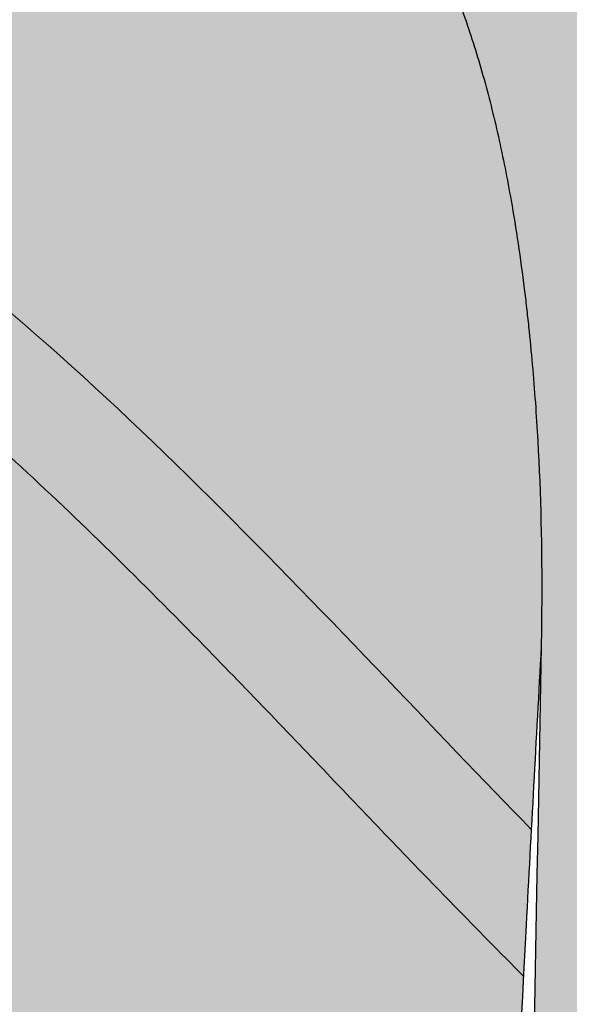
# Model space of a CAD drawing. Units: millimetres. Extents: x 11032 to 26788, y 3406 to 24505.
# Tile 60 of 78: x 16786 to 17293, y 16019 to 16927. Entities that reach past the tile are written whole.
import ezdxf

# ---------------------------------------------------------------- set-up
doc = ezdxf.new("R2010")
doc.units = ezdxf.units.MM
doc.header["$MEASUREMENT"] = 0
for name, color, linetype, lineweight in [('A-ANNO-DIMS', 2, 'Continuous', 18), ('A-ROOF', 7, 'Continuous', 30), ('E-LITE', 7, 'Continuous', 18), ('E-LITE-PATT', 7, 'Continuous', 13)]:
    doc.layers.add(name, color=color, linetype=linetype, lineweight=lineweight)
doc.layers.add('A-ROOF-PATT', color=9, linetype='Continuous', lineweight=13, true_color=0xc7c8ca)
doc.styles.get("Standard").update_dxf_attribs({"font": 'arial.ttf'})
doc.dimstyles.get("Standard").update_dxf_attribs({"dimtxt": 150, "dimasz": 100, "dimexe": 10, "dimexo": 5, "dimgap": 5, "dimtad": 0, "dimtih": 1, "dimtoh": 1, "dimdec": 0, "dimzin": 0, "dimdsep": 46, "dimtxsty": 'Standard', "dimcen": 0.09, "dimadec": 0, "dimazin": 0, "dimtfac": 1, "dimtdec": 0, "dimtofl": 0, "dimtmove": 0, "dimatfit": 3, "dimfxl": 1, "dimtolj": 1, "dimtzin": 0, "dimarcsym": 0})

# ---------------------------------------------------------------- blocks, each defined once
blk = doc.blocks.new('*D36')
at = {"layer": 'A-ANNO-DIMS', "color": 0, "lineweight": -2, "transparency": 16777216}
for p, q in [((12301.26, 17115.89), (12301.26, 24416.86)), ((25397.4, 4466.4), (25397.4, 24416.86)), ((12401.26, 24406.86), (18569.2, 24406.86)), ((25297.4, 24406.86), (19129.47, 24406.86))]:
    blk.add_line(p, q, dxfattribs=at)
at = {"layer": 'A-ANNO-DIMS', "color": 0, "transparency": 16777216}
for points in [[(12401.26, 24423.52), (12401.26, 24390.19), (12301.26, 24406.86)], [(25297.4, 24423.52), (25297.4, 24390.19), (25397.4, 24406.86)]]:
    blk.add_solid(points, dxfattribs=at)
at = {"layer": 'Defpoints', "color": 0, "transparency": 16777216}
for p in [(25397.4, 24406.86), (12301.26, 17110.89), (25397.4, 4461.4)]:
    blk.add_point(p, dxfattribs=at)
at = {"layer": 'A-ANNO-DIMS', "color": 0, "transparency": 16777216, "insert": (18849.33, 24406.86), "char_height": 150, "attachment_point": 5}
blk.add_mtext('\\A1;13096', dxfattribs=at)
blk = doc.blocks.new('*D37')
at = {"layer": 'A-ANNO-DIMS', "color": 0, "lineweight": -2, "transparency": 16777216}
for p, q in [((18087.74, 23450.36), (11334.76, 23450.36)), ((11344.76, 23350.36), (11344.76, 14037.46)), ((11344.76, 4561.4), (11344.76, 13874.29)), ((12927.66, 4461.4), (11334.76, 4461.4))]:
    blk.add_line(p, q, dxfattribs=at)
at = {"layer": 'A-ANNO-DIMS', "color": 0, "transparency": 16777216}
for points in [[(11328.1, 23350.36), (11361.43, 23350.36), (11344.76, 23450.36)], [(11328.1, 4561.4), (11361.43, 4561.4), (11344.76, 4461.4)]]:
    blk.add_solid(points, dxfattribs=at)
at = {"layer": 'Defpoints', "color": 0, "transparency": 16777216}
for p in [(11344.76, 23450.36), (18092.74, 23450.36), (12932.66, 4461.4)]:
    blk.add_point(p, dxfattribs=at)
at = {"layer": 'A-ANNO-DIMS', "color": 0, "transparency": 16777216, "insert": (11344.76, 13955.88), "char_height": 150, "attachment_point": 5}
blk.add_mtext('\\A1;18989', dxfattribs=at)
blk = doc.blocks.new('*D45')
at = {"layer": 'A-ANNO-DIMS', "color": 0, "lineweight": -2, "transparency": 16777216}
for p, q in [((13792.37, 18518.92), (26363.9, 18518.92)), ((26353.9, 18418.92), (26353.9, 17450.32)), ((26353.9, 16318.44), (26353.9, 17287.05)), ((22902.4, 16218.44), (26363.9, 16218.44))]:
    blk.add_line(p, q, dxfattribs=at)
at = {"layer": 'A-ANNO-DIMS', "color": 0, "transparency": 16777216}
for points in [[(26337.24, 18418.92), (26370.57, 18418.92), (26353.9, 18518.92)], [(26337.24, 16318.44), (26370.57, 16318.44), (26353.9, 16218.44)]]:
    blk.add_solid(points, dxfattribs=at)
at = {"layer": 'Defpoints', "color": 0, "transparency": 16777216}
for p in [(13787.37, 18518.92), (26353.9, 18518.92), (22897.4, 16218.44)]:
    blk.add_point(p, dxfattribs=at)
at = {"layer": 'A-ANNO-DIMS', "color": 0, "transparency": 16777216, "insert": (26353.9, 17368.68), "char_height": 150, "attachment_point": 5}
blk.add_mtext('\\A1;2300.5', dxfattribs=at)
blk = doc.blocks.new('*D57')
at = {"layer": 'A-ANNO-DIMS', "color": 0, "lineweight": -2, "transparency": 16777216}
for p, q in [((14994.7, 7266.4), (14994.7, 24416.86)), ((20894.7, 7266.4), (20894.7, 24416.86)), ((15094.7, 24406.86), (17715.98, 24406.86)), ((20794.7, 24406.86), (18173.42, 24406.86))]:
    blk.add_line(p, q, dxfattribs=at)
at = {"layer": 'A-ANNO-DIMS', "color": 0, "transparency": 16777216}
for points in [[(15094.7, 24423.52), (15094.7, 24390.19), (14994.7, 24406.86)], [(20794.7, 24423.52), (20794.7, 24390.19), (20894.7, 24406.86)]]:
    blk.add_solid(points, dxfattribs=at)
at = {"layer": 'Defpoints', "color": 0, "transparency": 16777216}
for p in [(20894.7, 24406.86), (14994.7, 7261.4), (20894.7, 7261.4)]:
    blk.add_point(p, dxfattribs=at)
at = {"layer": 'A-ANNO-DIMS', "color": 0, "transparency": 16777216, "insert": (17944.7, 24406.86), "char_height": 150, "attachment_point": 5}
blk.add_mtext('\\A1;5900', dxfattribs=at)

msp = doc.modelspace()

# ---------------------------------------------------------------- hatches: boundary and pattern name
at = {"layer": 'A-ROOF-PATT'}
h = msp.add_hatch(color=256, dxfattribs=at)
edge = h.paths.add_edge_path()
edge.add_spline(control_points=[(17532.827, 17324.837), (17391.335, 17349.016), (16840.872, 17494.912), (16080.055, 18069.544), (14738.803, 18299.641), (13382.429, 18838.336), (12580.532, 17870.207), (12430.422, 17563.822)], knot_values=[2977.6027945, 2977.6027945, 2977.6027945, 2977.6027945, 3438.1840601, 4811.6463022, 5622.8675483, 7588.0288188, 8560.6685791, 8560.6685791, 8560.6685791, 8560.6685791], degree=3, periodic=0)
edge.add_spline(control_points=[(12430.422, 17563.822), (12437.904, 17573.36), (12445.386, 17582.899), (12452.869, 17592.437), (12452.869, 17592.438), (12452.869, 17592.438), (12452.869, 17592.438)], knot_values=[1408.564138, 1408.564138, 1408.564138, 1408.564138, 1444.85989, 1444.85989, 1444.85989, 1444.8601183, 1444.8601183, 1444.8601183, 1444.8601183], degree=3, periodic=0)
edge.add_spline(control_points=[(12452.869, 17592.438), (12555.432, 17723.185), (12736.557, 17929.686), (13044.86, 18114.643), (13219.943, 18189.644), (13299.92, 18220.646)], knot_values=[339.318246, 339.318246, 339.318246, 339.318246, 836.8349967, 1151.2512933, 1408.564138, 1408.564138, 1408.564138, 1408.564138], degree=3, periodic=0)
edge.add_spline(control_points=[(13299.92, 18220.646), (13299.998, 18220.689), (13300.077, 18220.732), (13319.738, 18231.488), (13339.24, 18241.402), (13388.645, 18264.703), (13418.466, 18277.069), (13478.019, 18298.648), (13507.751, 18307.861), (13544.561, 18317.488), (13551.584, 18319.245), (13558.612, 18320.924)], knot_values=[3783.8950972, 3783.8950972, 3783.8950972, 3783.8950972, 3784.1737101, 3784.1737101, 3853.4666747, 3853.4666747, 3960.2401917, 3960.2401917, 4067.0137087, 4067.0137087, 4092.1744649, 4092.1744649, 4092.1744649, 4092.1744649], degree=3, periodic=0)
edge.add_spline(control_points=[(13558.612, 18320.924), (13581.407, 18326.373), (13604.25, 18331.007), (13657.184, 18339.957), (13687.338, 18343.732), (13748.098, 18348.892), (13778.704, 18350.276), (13840.46, 18350.833), (13871.609, 18350.005), (13934.496, 18346.313), (13966.232, 18343.449), (14030.297, 18335.871), (14062.625, 18331.158), (14127.853, 18320.088), (14160.753, 18313.73), (14241.357, 18296.556), (14289.343, 18284.997), (14386.31, 18259.688), (14435.291, 18245.941), (14534.161, 18217.034), (14584.049, 18201.875), (14684.682, 18170.964), (14735.427, 18155.212), (14837.763, 18123.971), (14889.354, 18108.482), (14954.971, 18089.677), (14968.586, 18085.823), (14992.391, 18079.184), (15002.566, 18076.376), (15021.739, 18071.153), (15030.731, 18068.729), (15047.707, 18064.21), (15055.694, 18062.106), (15079.815, 18055.825), (15095.905, 18051.728), (15143.966, 18039.717), (15175.729, 18032.084), (15254.84, 18013.501), (15301.798, 18002.866), (15394.186, 17981.845), (15439.615, 17971.459), (15528.833, 17950.135), (15572.62, 17939.197), (15658.477, 17916.021), (15700.546, 17903.785), (15753.633, 17886.734), (15765.446, 17882.835), (15786.574, 17875.653), (15795.915, 17872.404), (15810.108, 17867.349), (15814.99, 17865.588), (15824.736, 17862.029), (15829.611, 17860.226), (15844.241, 17854.75), (15854.002, 17851.008), (15883.312, 17839.521), (15902.885, 17831.512), (15966.355, 17804.548), (16010.39, 17784.302), (16098.838, 17741.267), (16143.25, 17718.478), (16232.497, 17671.098), (16277.332, 17646.507), (16367.515, 17596.295), (16412.862, 17570.676), (16504.202, 17519.209), (16550.194, 17493.362), (16643.009, 17442.263), (16689.831, 17417.011), (16756.517, 17382.472), (16775.937, 17372.58), (16795.455, 17362.84)], knot_values=[4092.1744649, 4092.1744649, 4092.1744649, 4092.1744649, 4173.7872258, 4173.7872258, 4280.5607428, 4280.5607428, 4387.3342598, 4387.3342598, 4494.1077768, 4494.1077768, 4600.8812939, 4600.8812939, 4707.6548109, 4707.6548109, 4814.4283279, 4814.4283279, 4967.1262405, 4967.1262405, 5119.8241531, 5119.8241531, 5272.5220657, 5272.5220657, 5425.2199783, 5425.2199783, 5577.9178908, 5577.9178908, 5617.7853319, 5617.7853319, 5647.4648479, 5647.4648479, 5673.611025, 5673.611025, 5696.747607, 5696.747607, 5743.6818903, 5743.6818903, 5837.5504571, 5837.5504571, 5979.7261046, 5979.7261046, 6121.9017521, 6121.9017521, 6264.0773996, 6264.0773996, 6406.2530471, 6406.2530471, 6447.2585849, 6447.2585849, 6480.0420882, 6480.0420882, 6497.3077062, 6497.3077062, 6514.5733242, 6514.5733242, 6549.1045602, 6549.1045602, 6618.1670322, 6618.1670322, 6772.6610171, 6772.6610171, 6927.155002, 6927.155002, 7081.6489869, 7081.6489869, 7236.1429718, 7236.1429718, 7390.6369567, 7390.6369567, 7545.1309416, 7545.1309416, 7608.1992868, 7608.1992868, 7608.1992868, 7608.1992868], degree=3, periodic=0)
edge.add_spline(control_points=[(16795.455, 17362.84), (16814.335, 17349.456), (16832.897, 17336.263), (16873.225, 17307.197), (16894.778, 17291.386), (16936.221, 17259.941), (16956.11, 17244.308), (16993.863, 17213.094), (17011.726, 17197.514), (17041.993, 17169.265), (17054.791, 17156.601), (17078.762, 17131.225), (17089.933, 17118.516), (17110.618, 17092.991), (17120.131, 17080.178), (17130.17, 17065.264), (17131.487, 17063.277), (17133.77, 17059.776), (17134.746, 17058.261), (17136.69, 17055.205), (17137.657, 17053.668), (17140.539, 17049.025), (17142.438, 17045.89), (17148.068, 17036.367), (17151.732, 17029.859), (17163.03, 17008.788), (17170.335, 16993.646), (17184.087, 16961.978), (17190.534, 16945.453), (17202.562, 16911.165), (17208.142, 16893.402), (17218.448, 16856.821), (17223.173, 16838.003), (17231.801, 16799.51), (17235.705, 16779.837), (17241.533, 16746.739), (17243.676, 16733.5), (17247.718, 16706.37), (17249.608, 16692.472), (17252.066, 16672.69), (17252.761, 16666.875), (17254.1, 16655.226), (17254.744, 16649.4), (17256.596, 16631.917), (17257.727, 16620.254), (17260.823, 16585.238), (17262.489, 16561.858), (17266.551, 16488.654), (17267.658, 16438.661), (17267.349, 16375.228), (17267.193, 16362.07), (17266.95, 16348.891)], knot_values=[15.1130472, 15.1130472, 15.1130472, 15.1130472, 82.6995146, 82.6995146, 165.3990291, 165.3990291, 248.0985437, 248.0985437, 330.7980583, 330.7980583, 397.9419458, 397.9419458, 465.0858333, 465.0858333, 532.2297209, 532.2297209, 542.533741, 542.533741, 550.3568158, 550.3568158, 558.1798906, 558.1798906, 573.8260402, 573.8260402, 605.1183395, 605.1183395, 672.7640614, 672.7640614, 740.4097834, 740.4097834, 808.0555054, 808.0555054, 875.7012273, 875.7012273, 943.3469493, 943.3469493, 987.6613492, 987.6613492, 1033.4121612, 1033.4121612, 1052.3850876, 1052.3850876, 1071.358014, 1071.358014, 1109.3038668, 1109.3038668, 1185.1955724, 1185.1955724, 1346.4419026, 1346.4419026, 1388.5586631, 1388.5586631, 1388.5586631, 1388.5586631], degree=3, periodic=0)
edge.add_spline(control_points=[(17266.95, 16348.891), (17266.95, 16348.891), (17266.95, 16348.891), (17266.95, 16348.891), (17253.182, 15602.417), (17239.414, 14855.943), (17225.646, 14109.469)], knot_values=[1388.5586631, 1388.5586631, 1388.5586631, 1388.5586631, 1388.5589654, 1388.5589654, 1388.5589654, 3774.0767661, 3774.0767661, 3774.0767661, 3774.0767661], degree=3, periodic=0)
edge.add_spline(control_points=[(17225.646, 14109.469), (17226.198, 14109.827), (17226.748, 14110.185), (17242.065, 14120.191), (17255.956, 14130.116), (17274.422, 14144.286), (17279.609, 14148.386), (17284.686, 14152.511)], knot_values=[1926.3423968, 1926.3423968, 1926.3423968, 1926.3423968, 1927.316729, 1927.316729, 1953.5121761, 1953.5121761, 1964.0732348, 1964.0732348, 1964.0732348, 1964.0732348], degree=3, periodic=0)
edge.add_spline(control_points=[(17284.686, 14152.511), (17315.791, 14194.761), (17384.413, 14446.273), (17407.128, 14793.401), (17407.093, 15295.84), (17423.274, 15626.362), (17415.601, 15782.507)], knot_values=[0, 0, 0, 0, 163.2554674, 619.2296767, 1171.8624483, 1621.6355562, 1621.6355562, 1621.6355562, 1621.6355562], degree=3, periodic=0)
edge.add_spline(control_points=[(17415.601, 15782.507), (17438.21, 16077.57), (17410.495, 16533.484), (17390.893, 17030.649), (17301.082, 17169.349)], knot_values=[543.9784753, 543.9784753, 543.9784753, 543.9784753, 1452.9852767, 1960.0114926, 1960.0114926, 1960.0114926, 1960.0114926], degree=3, periodic=0)
edge.add_spline(control_points=[(17301.082, 17169.349), (17346.58, 17157.64), (17392.235, 17147.336), (17467.161, 17132.609), (17496.336, 17127.412), (17525.58, 17122.709)], knot_values=[8131.593939, 8131.593939, 8131.593939, 8131.593939, 8269.7349273, 8269.7349273, 8357.5016646, 8357.5016646, 8357.5016646, 8357.5016646], degree=3, periodic=0)
edge.add_line((17525.58, 17122.709), (17532.827, 17324.837))
edge = h.paths.add_edge_path(flags=17)
edge.add_spline(control_points=[(13340.537, 14602.706), (13316.172, 14726.456), (13323.666, 14932.342), (13637.836, 15081.117), (13863.248, 15171.051), (14002.1, 15224.503), (14058.539, 15244.876)], knot_values=[680.8931862, 680.8931862, 680.8931862, 680.8931862, 1033.4728289, 1337.4008326, 1604.7214264, 1784.2944722, 1784.2944722, 1784.2944722, 1784.2944722], degree=3, periodic=0)
edge.add_spline(control_points=[(14058.539, 15244.876), (14058.289, 15275.236), (14057.634, 15305.434), (14055.312, 15376.527), (14053.359, 15417.248), (14048.642, 15497.048), (14045.89, 15536.143), (14042.888, 15574.619)], knot_values=[6573.1065419, 6573.1065419, 6573.1065419, 6573.1065419, 6636.7330012, 6636.7330012, 6723.8890547, 6723.8890547, 6809.6328771, 6809.6328771, 6809.6328771, 6809.6328771], degree=3, periodic=0)
edge.add_spline(control_points=[(14042.888, 15574.619), (13546.54, 15403.221), (13074.735, 15143.241), (13277.36, 14695.339), (13340.537, 14602.706)], knot_values=[503.7925783, 503.7925783, 503.7925783, 503.7925783, 1728.1787606, 2051.34844, 2051.34844, 2051.34844, 2051.34844], degree=3, periodic=0)
h = msp.add_hatch(color=256, dxfattribs=at)
h.set_gradient(color1=(254, 234, 185), color2=(254, 204, 102), name='HEMISPHERICAL')
edge = h.paths.add_edge_path()
edge.add_line((15084.393, 17001.32), (15284.393, 17051.32))
edge.add_line((15284.393, 17051.32), (15470.537, 16752.334))
edge.add_spline(control_points=[(15470.537, 16752.334), (15683.311, 16831.508), (16106.827, 16912.335), (16625.609, 16876.997), (17083.498, 16357.78), (17257.801, 16180.113)], knot_values=[0, 0, 0, 0, 655.2936334, 1252.0157838, 1989.6162859, 1989.6162859, 1989.6162859, 1989.6162859], degree=3, periodic=0)
edge.add_spline(control_points=[(17257.801, 16180.113), (17260.851, 16236.372), (17263.9, 16292.632), (17266.95, 16348.891)], knot_values=[1132.9967717, 1132.9967717, 1132.9967717, 1132.9967717, 1198.0464225, 1198.0464225, 1198.0464225, 1198.0464225], degree=3, periodic=0)
edge.add_spline(control_points=[(17266.95, 16348.891), (17267.193, 16362.07), (17267.349, 16375.228), (17267.658, 16438.661), (17266.551, 16488.654), (17262.489, 16561.858), (17260.823, 16585.238), (17257.727, 16620.254), (17256.596, 16631.917), (17254.744, 16649.4), (17254.1, 16655.226), (17252.761, 16666.875), (17252.066, 16672.69), (17249.608, 16692.472), (17247.718, 16706.37), (17243.676, 16733.5), (17241.533, 16746.739), (17235.705, 16779.837), (17231.801, 16799.51), (17223.173, 16838.003), (17218.448, 16856.821), (17208.142, 16893.402), (17202.562, 16911.165), (17190.534, 16945.453), (17184.087, 16961.978), (17170.335, 16993.646), (17163.03, 17008.788), (17151.732, 17029.859), (17148.068, 17036.367), (17142.438, 17045.89), (17140.539, 17049.025), (17137.657, 17053.668), (17136.69, 17055.205), (17134.746, 17058.261), (17133.77, 17059.776), (17131.487, 17063.277), (17130.17, 17065.264), (17120.131, 17080.178), (17110.618, 17092.991), (17089.933, 17118.516), (17078.762, 17131.225), (17054.791, 17156.601), (17041.993, 17169.265), (17011.726, 17197.514), (16993.863, 17213.094), (16956.11, 17244.308), (16936.221, 17259.941), (16894.778, 17291.386), (16873.225, 17307.197), (16832.897, 17336.263), (16814.335, 17349.456), (16795.455, 17362.84)], knot_values=[15.1130472, 15.1130472, 15.1130472, 15.1130472, 57.2298077, 57.2298077, 218.4761379, 218.4761379, 294.3678435, 294.3678435, 332.3136963, 332.3136963, 351.2866227, 351.2866227, 370.2595491, 370.2595491, 416.0103612, 416.0103612, 460.324761, 460.324761, 527.970483, 527.970483, 595.616205, 595.616205, 663.2619269, 663.2619269, 730.9076489, 730.9076489, 798.5533709, 798.5533709, 829.8456701, 829.8456701, 845.4918197, 845.4918197, 853.3148945, 853.3148945, 861.1379693, 861.1379693, 871.4419895, 871.4419895, 938.585877, 938.585877, 1005.7297645, 1005.7297645, 1072.8736521, 1072.8736521, 1155.5731666, 1155.5731666, 1238.2726812, 1238.2726812, 1320.9721958, 1320.9721958, 1388.5586631, 1388.5586631, 1388.5586631, 1388.5586631], degree=3, periodic=0)
edge.add_spline(control_points=[(16795.455, 17362.84), (16775.937, 17372.58), (16756.517, 17382.472), (16689.831, 17417.011), (16643.009, 17442.263), (16550.194, 17493.362), (16504.202, 17519.209), (16412.862, 17570.676), (16367.515, 17596.295), (16277.332, 17646.507), (16232.497, 17671.098), (16143.25, 17718.478), (16098.838, 17741.267), (16010.39, 17784.302), (15966.355, 17804.548), (15902.885, 17831.512), (15883.312, 17839.521), (15854.002, 17851.008), (15844.241, 17854.75), (15829.611, 17860.226), (15824.736, 17862.029), (15814.99, 17865.588), (15810.108, 17867.349), (15795.915, 17872.404), (15786.574, 17875.653), (15765.446, 17882.835), (15753.633, 17886.734), (15700.546, 17903.785), (15658.477, 17916.021), (15572.62, 17939.197), (15528.833, 17950.135), (15439.615, 17971.459), (15394.186, 17981.845), (15301.798, 18002.866), (15254.84, 18013.501), (15175.729, 18032.084), (15143.966, 18039.717), (15095.905, 18051.728), (15079.815, 18055.825), (15055.694, 18062.106), (15047.707, 18064.21), (15030.731, 18068.729), (15021.739, 18071.153), (15002.566, 18076.376), (14992.391, 18079.184), (14968.586, 18085.823), (14954.971, 18089.677), (14889.354, 18108.482), (14837.763, 18123.971), (14735.427, 18155.212), (14684.682, 18170.964), (14584.049, 18201.875), (14534.161, 18217.034), (14435.291, 18245.941), (14386.31, 18259.688), (14289.343, 18284.997), (14241.357, 18296.556), (14160.753, 18313.73), (14127.853, 18320.088), (14062.625, 18331.158), (14030.297, 18335.871), (13966.232, 18343.449), (13934.496, 18346.313), (13871.609, 18350.005), (13840.46, 18350.833), (13778.704, 18350.276), (13748.098, 18348.892), (13687.338, 18343.732), (13657.184, 18339.957), (13604.25, 18331.007), (13581.407, 18326.373), (13558.612, 18320.924)], knot_values=[4092.1744649, 4092.1744649, 4092.1744649, 4092.1744649, 4155.2428101, 4155.2428101, 4309.736795, 4309.736795, 4464.2307799, 4464.2307799, 4618.7247648, 4618.7247648, 4773.2187497, 4773.2187497, 4927.7127346, 4927.7127346, 5082.2067195, 5082.2067195, 5151.2691915, 5151.2691915, 5185.8004275, 5185.8004275, 5203.0660455, 5203.0660455, 5220.3316635, 5220.3316635, 5253.1151668, 5253.1151668, 5294.1207046, 5294.1207046, 5436.2963521, 5436.2963521, 5578.4719996, 5578.4719996, 5720.6476471, 5720.6476471, 5862.8232946, 5862.8232946, 5956.6918614, 5956.6918614, 6003.6261447, 6003.6261447, 6026.7627267, 6026.7627267, 6052.9089038, 6052.9089038, 6082.5884198, 6082.5884198, 6122.4558609, 6122.4558609, 6275.1537734, 6275.1537734, 6427.851686, 6427.851686, 6580.5495986, 6580.5495986, 6733.2475112, 6733.2475112, 6885.9454238, 6885.9454238, 6992.7189408, 6992.7189408, 7099.4924578, 7099.4924578, 7206.2659749, 7206.2659749, 7313.0394919, 7313.0394919, 7419.8130089, 7419.8130089, 7526.5865259, 7526.5865259, 7608.1992868, 7608.1992868, 7608.1992868, 7608.1992868], degree=3, periodic=0)
edge.add_spline(control_points=[(13558.612, 18320.924), (13472.381, 18287.498), (13386.15, 18254.072), (13299.92, 18220.646), (13299.92, 18220.646), (13299.92, 18220.646), (13299.92, 18220.646)], knot_values=[61.8832457, 61.8832457, 61.8832457, 61.8832457, 339.3179746, 339.3179746, 339.3179746, 339.318246, 339.318246, 339.318246, 339.318246], degree=3, periodic=0)
edge.add_spline(control_points=[(13299.92, 18220.646), (13219.943, 18189.644), (13044.86, 18114.643), (12736.557, 17929.686), (12555.432, 17723.185), (12452.869, 17592.438)], knot_values=[339.318246, 339.318246, 339.318246, 339.318246, 596.6310906, 911.0473872, 1408.564138, 1408.564138, 1408.564138, 1408.564138], degree=3, periodic=0)
edge.add_spline(control_points=[(12452.869, 17592.438), (12452.869, 17592.438), (12452.869, 17592.438), (12452.869, 17592.437), (12445.386, 17582.899), (12437.904, 17573.36), (12430.422, 17563.822)], knot_values=[1408.564138, 1408.564138, 1408.564138, 1408.564138, 1408.5643663, 1408.5643663, 1408.5643663, 1444.8601183, 1444.8601183, 1444.8601183, 1444.8601183], degree=3, periodic=0)
edge.add_spline(control_points=[(12430.422, 17563.822), (12373.797, 17448.248), (12157.302, 16836.764), (12751.985, 16393.69), (13424.325, 15907.903), (14042.888, 15574.619)], knot_values=[0, 0, 0, 0, 366.8993034, 1975.5941082, 2977.6027945, 2977.6027945, 2977.6027945, 2977.6027945], degree=3, periodic=0)
edge.add_spline(control_points=[(14042.888, 15574.619), (14042.839, 15575.252), (14042.789, 15575.886), (14039.681, 15615.607), (14036.366, 15654.052), (14029.551, 15729.305), (14026.05, 15766.114), (14019.175, 15837.686), (14015.8, 15872.45), (13903.823, 16338.596)], knot_values=[6310.2261504, 6310.2261504, 6310.2261504, 6310.2261504, 6311.6383814, 6311.6383814, 6398.7944349, 6398.7944349, 6485.9504884, 6485.9504884, 6573.1065419, 6573.1065419, 6573.1065419, 6573.1065419], degree=3, periodic=0)
edge.add_spline(control_points=[(13903.823, 16338.596), (14237.315, 16236.889), (14456.623, 16167.555), (14614.196, 16115.84)], knot_values=[0, 0, 0, 0, 202.9853419, 202.9853419, 202.9853419, 202.9853419], degree=3, periodic=0)
edge.add_spline(control_points=[(14614.196, 16115.84), (14663.209, 16178.992), (14799.965, 16341.237), (14969.915, 16481.426), (15084.393, 16556.825)], knot_values=[2405.0345045, 2405.0345045, 2405.0345045, 2405.0345045, 2644.8826966, 3039.2707272, 3039.2707272, 3039.2707272, 3039.2707272], degree=3, periodic=0)
edge.add_line((15084.393, 16556.825), (15084.393, 17001.32))
h.paths.add_polyline_path([(14195.599, 17606.181, -1), (14395.599, 17606.181, -1)], flags=16)
h.paths.add_polyline_path([(13310.178, 17032.97, -1), (13510.178, 17032.97, -1)], flags=16)
h = msp.add_hatch(color=256, dxfattribs=at)
h.set_gradient(color1=(254, 234, 185), color2=(254, 204, 102), name='HEMISPHERICAL')
edge = h.paths.add_edge_path()
edge.add_spline(control_points=[(16560.042, 14907.752), (16569.192, 14907.664), (16578.343, 14907.575), (16587.493, 14907.486), (16832.101, 14905.115), (17122.895, 14902.296), (16849.359, 14976.117), (16870.954, 15304.114), (17098.337, 15241.178), (17235.385, 15203.245)], knot_values=[0, 0, 0, 0, 14.8674385, 14.8674385, 14.8674385, 412.2943091, 487.3345915, 708.6416004, 1044.3939449, 1044.3939449, 1044.3939449, 1044.3939449], degree=3, periodic=0)
edge.add_line((16587.504, 14907.486), (16560.207, 14907.486))
edge.add_line((16560.207, 14907.486), (15784.393, 16153.61))
edge.add_line((15784.393, 16153.61), (15784.393, 15385.996))
edge.add_spline(control_points=[(15784.393, 15385.996), (15798.391, 15360.52), (15847.198, 15266.214), (15887.196, 15168.614), (15912.903, 15096.727)], knot_values=[1463.2850479, 1463.2850479, 1463.2850479, 1463.2850479, 1550.659771, 1779.9599361, 1779.9599361, 1779.9599361, 1779.9599361], degree=3, periodic=0)
edge.add_spline(control_points=[(15912.903, 15096.727), (15913.652, 15095.649), (15914.403, 15094.565), (15925.191, 15078.948), (15935.516, 15063.47), (15956.582, 15030.918), (15967.324, 15013.844), (15989.119, 14978.386), (16000.173, 14960.003), (16022.525, 14922.193), (16033.824, 14902.767), (16056.63, 14863.116), (16068.138, 14842.891), (16091.349, 14801.871), (16103.053, 14781.075), (16126.666, 14739.118), (16138.575, 14717.958), (16162.628, 14675.459), (16174.772, 14654.12), (16199.352, 14611.428), (16211.787, 14590.075), (16237.037, 14547.491), (16249.851, 14526.26), (16271.946, 14490.566), (16281.092, 14476.044), (16299.694, 14447.129), (16309.149, 14432.737), (16328.456, 14404.098), (16338.307, 14389.85), (16358.518, 14361.503), (16368.879, 14347.403), (16390.266, 14319.347), (16401.291, 14305.391), (16420.626, 14281.969), (16428.703, 14272.467), (16445.363, 14253.527), (16453.946, 14244.088), (16471.727, 14225.278), (16480.926, 14215.907), (16500.075, 14197.247), (16510.026, 14187.959), (16530.844, 14169.504), (16541.71, 14160.337), (16564.549, 14142.195), (16576.522, 14133.22), (16597.69, 14118.448), (16606.528, 14112.565), (16624.87, 14101.004), (16634.376, 14095.326), (16654.117, 14084.255), (16664.352, 14078.862), (16685.603, 14068.46), (16696.619, 14063.452), (16719.46, 14053.944), (16731.285, 14049.444), (16755.742, 14041.097), (16768.374, 14037.251), (16794.396, 14030.368), (16807.787, 14027.332), (16835.229, 14022.23), (16849.279, 14020.163), (16877.882, 14017.141), (16892.435, 14016.186), (16921.835, 14015.489), (16936.683, 14015.749), (16961.564, 14017.241), (16971.582, 14018.127), (16986.57, 14019.883), (16991.56, 14020.54), (16999.027, 14021.63), (17001.514, 14022.011), (17006.48, 14022.809), (17008.962, 14023.225), (17014.824, 14024.251), (17018.193, 14024.875), (17036.262, 14028.398), (17050.55, 14031.826), (17078.171, 14039.583), (17091.505, 14043.912), (17115.643, 14052.705), (17126.557, 14057.089), (17137.108, 14061.688)], knot_values=[2010.7639617, 2010.7639617, 2010.7639617, 2010.7639617, 2014.7029827, 2014.7029827, 2067.238337, 2067.238337, 2119.7736913, 2119.7736913, 2172.3090457, 2172.3090457, 2224.8444, 2224.8444, 2277.3797543, 2277.3797543, 2329.9151086, 2329.9151086, 2382.450463, 2382.450463, 2434.9858173, 2434.9858173, 2487.5211716, 2487.5211716, 2540.0565259, 2540.0565259, 2576.3179289, 2576.3179289, 2612.5793318, 2612.5793318, 2648.8407347, 2648.8407347, 2685.1021376, 2685.1021376, 2721.3635405, 2721.3635405, 2746.252015, 2746.252015, 2771.1404895, 2771.1404895, 2796.028964, 2796.028964, 2820.9174385, 2820.9174385, 2845.8059131, 2845.8059131, 2870.6943876, 2870.6943876, 2887.5132757, 2887.5132757, 2904.3321639, 2904.3321639, 2921.1510521, 2921.1510521, 2937.9699402, 2937.9699402, 2954.7888284, 2954.7888284, 2971.6077166, 2971.6077166, 2988.4266047, 2988.4266047, 3005.2454929, 3005.2454929, 3022.0643811, 3022.0643811, 3038.8832692, 3038.8832692, 3050.1975453, 3050.1975453, 3055.8546833, 3055.8546833, 3058.6832524, 3058.6832524, 3061.5118214, 3061.5118214, 3065.3934173, 3065.3934173, 3082.4668716, 3082.4668716, 3099.5403259, 3099.5403259, 3114.5433443, 3114.5433443, 3114.5433443, 3114.5433443], degree=3, periodic=0)
edge.add_spline(control_points=[(17137.108, 14061.688), (17165.253, 14274.398), (17209.97, 14653.885), (17230.2, 15035.586), (17235.385, 15203.245)], knot_values=[1968.0804557, 1968.0804557, 1968.0804557, 1968.0804557, 2611.5282875, 3114.5379264, 3114.5379264, 3114.5379264, 3114.5379264], degree=3, periodic=0)
edge = h.paths.add_edge_path()
edge.add_spline(control_points=[(16856.103, 14956.992), (16852.841, 14961.219), (16849.83, 14965.576), (16842.539, 14977.287), (16838.658, 14984.798), (16832.033, 15000.109), (16829.289, 15007.911), (16824.126, 15026.008), (16822.047, 15036.354), (16819.308, 15057.097), (16818.649, 15067.496), (16818.576, 15088.188), (16819.162, 15098.483), (16821.467, 15118.823), (16823.186, 15128.868), (16827.696, 15148.567), (16830.486, 15158.22), (16836.065, 15173.969), (16838.565, 15180.211), (16844.079, 15192.402), (16847.092, 15198.353), (16852.029, 15207.021), (16853.744, 15209.868), (16857.321, 15215.468), (16859.188, 15218.226), (16863.017, 15223.558), (16864.978, 15226.136), (16872.565, 15235.558), (16878.593, 15241.952), (16891.428, 15253.591), (16898.232, 15258.834), (16912.397, 15268.127), (16919.756, 15272.176), (16934.816, 15279.138), (16942.515, 15282.052), (16958.1, 15286.873), (16965.985, 15288.78), (16984.013, 15292.142), (16994.186, 15293.334), (17014.631, 15294.619), (17024.904, 15294.713), (17048.453, 15293.935), (17061.76, 15292.783), (17088.519, 15289.422), (17101.972, 15287.211), (17131.961, 15281.46), (17148.526, 15277.734), (17181.692, 15269.627), (17198.292, 15265.245), (17222.182, 15258.759), (17229.535, 15256.737), (17236.862, 15254.714)], knot_values=[9.6639535, 9.6639535, 9.6639535, 9.6639535, 20.0351668, 20.0351668, 36.9411752, 36.9411752, 53.8471837, 53.8471837, 75.7795687, 75.7795687, 97.7119538, 97.7119538, 119.6443388, 119.6443388, 141.5767238, 141.5767238, 163.5091089, 163.5091089, 178.3829945, 178.3829945, 193.2568801, 193.2568801, 200.6938229, 200.6938229, 208.1307657, 208.1307657, 215.4448585, 215.4448585, 235.5795923, 235.5795923, 255.7143261, 255.7143261, 275.8490598, 275.8490598, 295.9837936, 295.9837936, 316.1185274, 316.1185274, 341.7220543, 341.7220543, 367.3255812, 367.3255812, 400.1572431, 400.1572431, 432.988905, 432.988905, 473.0440165, 473.0440165, 513.099128, 513.099128, 530.9692999, 530.9692999, 530.9692999, 530.9692999], degree=3, periodic=0)
edge.add_spline(control_points=[(17236.862, 15254.714), (17240.377, 15387.456), (17242.496, 15609.536), (17239.752, 15831.567), (17250.544, 16044.717)], knot_values=[1250.9818616, 1250.9818616, 1250.9818616, 1250.9818616, 1649.1516581, 1916.613987, 1916.613987, 1916.613987, 1916.613987], degree=3, periodic=0)
edge.add_spline(control_points=[(17250.544, 16044.717), (17229.169, 16066.505), (17207.794, 16088.292), (17186.419, 16110.08), (17186.418, 16110.08), (17186.418, 16110.081), (17186.418, 16110.081)], knot_values=[-88.5185581, -88.5185581, -88.5185581, -88.5185581, -0.0012784, -0.0012784, -0.0012784, 0, 0, 0, 0], degree=3, periodic=0)
edge.add_spline(control_points=[(17186.418, 16110.081), (17169.261, 16127.569), (17151.499, 16145.947), (17114.892, 16184.084), (17096.046, 16203.842), (17057.437, 16244.305), (17037.673, 16265.01), (16997.415, 16306.918), (16976.921, 16328.12), (16927.79, 16378.347), (16898.924, 16407.388), (16840.771, 16464.327), (16811.484, 16492.225), (16758.449, 16540.764), (16734.666, 16561.798), (16687.634, 16601.588), (16664.382, 16620.344), (16624.116, 16650.909), (16606.897, 16663.324), (16583.769, 16678.999), (16577.49, 16683.149), (16567.144, 16689.805), (16563.039, 16692.397), (16550.823, 16699.959), (16542.775, 16704.739), (16526.841, 16713.814), (16518.956, 16718.108), (16495.524, 16730.301), (16480.199, 16737.514), (16449.97, 16750.334), (16435.066, 16755.942), (16405.476, 16765.764), (16390.79, 16769.979), (16361.418, 16777.195), (16346.731, 16780.197), (16317.147, 16785.133), (16302.249, 16787.067), (16272.053, 16789.992), (16256.756, 16790.981), (16225.609, 16792.125), (16209.759, 16792.279), (16177.385, 16791.865), (16160.862, 16791.296), (16136.98, 16790.07), (16129.942, 16789.661), (16118.22, 16788.91), (16113.574, 16788.594), (16103.645, 16787.886), (16098.362, 16787.489), (16087.761, 16786.652), (16082.439, 16786.212), (16066.413, 16784.825), (16055.649, 16783.812), (16023.135, 16780.505), (16001.164, 16777.942), (15934.539, 16769.141), (15889.17, 16761.791), (15797.417, 16743.949), (15751.033, 16733.457), (15645.217, 16705.796), (15585.74, 16687.58), (15526.207, 16666.217), (15525.367, 16665.915), (15524.528, 16665.613)], knot_values=[0, 0, 0, 0, 71.0501454, 71.0501454, 142.1002909, 142.1002909, 213.1504363, 213.1504363, 284.2005818, 284.2005818, 381.323193, 381.323193, 478.4458043, 478.4458043, 557.8219847, 557.8219847, 637.1981651, 637.1981651, 698.3122593, 698.3122593, 721.3971375, 721.3971375, 736.7790891, 736.7790891, 767.5429924, 767.5429924, 798.3068957, 798.3068957, 859.8347022, 859.8347022, 921.3625088, 921.3625088, 982.8903154, 982.8903154, 1044.4181219, 1044.4181219, 1105.9459285, 1105.9459285, 1167.4737351, 1167.4737351, 1229.0015416, 1229.0015416, 1290.5293482, 1290.5293482, 1315.8990035, 1315.8990035, 1332.3812792, 1332.3812792, 1350.9052657, 1350.9052657, 1369.4292522, 1369.4292522, 1406.4772252, 1406.4772252, 1480.5731712, 1480.5731712, 1628.7650633, 1628.7650633, 1776.9569554, 1776.9569554, 1966.3109251, 1966.3109251, 1969.019495, 1969.019495, 1969.019495, 1969.019495], degree=3, periodic=0)
edge.add_line((15524.528, 16665.613), (16587.978, 14957.484))
edge.add_spline(control_points=[(16587.978, 14957.484), (16605.253, 14957.316), (16622.516, 14957.149), (16665.945, 14956.759), (16691.933, 14956.554), (16742.419, 14956.302), (16766.918, 14956.255), (16813.531, 14956.412), (16835.647, 14956.617), (16856.103, 14956.992)], knot_values=[872.2181925, 872.2181925, 872.2181925, 872.2181925, 900.2857301, 900.2857301, 943.3659889, 943.3659889, 986.4462476, 986.4462476, 1029.5265064, 1029.5265064, 1029.5265064, 1029.5265064], degree=3, periodic=0)
h.paths.add_polyline_path([(16474.605, 15622.642, -1), (16624.605, 15622.642, -1)], flags=16)
h.paths.add_polyline_path([(16198.536, 16037.613, -1), (16348.536, 16037.613, -1)], flags=16)
h.paths.add_polyline_path([(16475.717, 16408.125, -1), (16625.717, 16408.125, -1)], flags=16)
at = {"layer": 'E-LITE-PATT'}
h = msp.add_hatch(color=256, dxfattribs=at)
edge = h.paths.add_edge_path()
edge.add_spline(control_points=[(15084.393, 16556.825), (14969.915, 16481.426), (14799.965, 16341.237), (14663.209, 16178.992), (14614.196, 16115.84)], knot_values=[2405.0345045, 2405.0345045, 2405.0345045, 2405.0345045, 2799.422535, 3039.2707272, 3039.2707272, 3039.2707272, 3039.2707272], degree=3, periodic=0)
edge.add_spline(control_points=[(14614.196, 16115.84), (14650.957, 16103.776), (14684.357, 16092.67), (14715.064, 16082.336)], knot_values=[202.9853419, 202.9853419, 202.9853419, 202.9853419, 250.3408615, 250.3408615, 250.3408615, 250.3408615], degree=3, periodic=0)
edge.add_spline(control_points=[(14715.064, 16082.336), (14732.32, 16103.979), (14749.873, 16125.274), (14780.086, 16160.475), (14792.544, 16174.592), (14817.876, 16202.424), (14830.748, 16216.137), (14853.903, 16239.975), (14864.109, 16250.213), (14884.415, 16270.066), (14894.503, 16279.688), (14918.667, 16302.183), (14932.865, 16314.967), (14987.375, 16362.454), (15029.339, 16395.81), (15076.718, 16430.13), (15080.55, 16432.882), (15084.393, 16435.621)], knot_values=[2472.5855096, 2472.5855096, 2472.5855096, 2472.5855096, 2558.786533, 2558.786533, 2617.7975153, 2617.7975153, 2676.8084975, 2676.8084975, 2721.9976237, 2721.9976237, 2765.3424393, 2765.3424393, 2824.4059302, 2824.4059302, 2988.2351723, 2988.2351723, 3002.5987883, 3002.5987883, 3002.5987883, 3002.5987883], degree=3, periodic=0)
edge.add_line((15084.393, 16435.621), (15084.393, 16556.825))
edge = h.paths.add_edge_path()
edge.add_spline(control_points=[(17257.801, 16180.113), (17083.498, 16357.78), (16625.609, 16876.997), (16106.827, 16912.335), (15683.311, 16831.508), (15470.537, 16752.334)], knot_values=[0, 0, 0, 0, 737.600502, 1334.3226525, 1989.6162859, 1989.6162859, 1989.6162859, 1989.6162859], degree=3, periodic=0)
edge.add_line((15470.537, 16752.334), (15524.528, 16665.613))
edge.add_spline(control_points=[(15524.528, 16665.613), (15525.367, 16665.915), (15526.207, 16666.217), (15585.74, 16687.58), (15645.217, 16705.796), (15751.033, 16733.457), (15797.417, 16743.949), (15889.17, 16761.791), (15934.539, 16769.141), (16001.164, 16777.942), (16023.135, 16780.505), (16055.649, 16783.812), (16066.413, 16784.825), (16082.439, 16786.212), (16087.761, 16786.652), (16098.362, 16787.489), (16103.645, 16787.886), (16113.574, 16788.594), (16118.22, 16788.91), (16129.942, 16789.661), (16136.98, 16790.07), (16160.862, 16791.296), (16177.385, 16791.865), (16209.759, 16792.279), (16225.609, 16792.125), (16256.756, 16790.981), (16272.053, 16789.992), (16302.249, 16787.067), (16317.147, 16785.133), (16346.731, 16780.197), (16361.418, 16777.195), (16390.79, 16769.979), (16405.476, 16765.764), (16435.066, 16755.942), (16449.97, 16750.334), (16480.199, 16737.514), (16495.524, 16730.301), (16518.956, 16718.108), (16526.841, 16713.814), (16542.775, 16704.739), (16550.823, 16699.959), (16563.039, 16692.397), (16567.144, 16689.805), (16577.49, 16683.149), (16583.769, 16678.999), (16606.897, 16663.324), (16624.116, 16650.909), (16664.382, 16620.344), (16687.634, 16601.588), (16734.666, 16561.798), (16758.449, 16540.764), (16811.484, 16492.225), (16840.771, 16464.327), (16898.924, 16407.388), (16927.79, 16378.347), (16976.921, 16328.12), (16997.415, 16306.918), (17037.673, 16265.01), (17057.437, 16244.305), (17096.046, 16203.842), (17114.892, 16184.084), (17151.499, 16145.947), (17169.261, 16127.569), (17186.418, 16110.081)], knot_values=[0, 0, 0, 0, 2.7085699, 2.7085699, 192.0625397, 192.0625397, 340.2544317, 340.2544317, 488.4463238, 488.4463238, 562.5422698, 562.5422698, 599.5902428, 599.5902428, 618.1142294, 618.1142294, 636.6382159, 636.6382159, 653.1204915, 653.1204915, 678.4901469, 678.4901469, 740.0179534, 740.0179534, 801.54576, 801.54576, 863.0735665, 863.0735665, 924.6013731, 924.6013731, 986.1291797, 986.1291797, 1047.6569862, 1047.6569862, 1109.1847928, 1109.1847928, 1170.7125993, 1170.7125993, 1201.4765026, 1201.4765026, 1232.2404059, 1232.2404059, 1247.6223576, 1247.6223576, 1270.7072358, 1270.7072358, 1331.8213299, 1331.8213299, 1411.1975103, 1411.1975103, 1490.5736908, 1490.5736908, 1587.696302, 1587.696302, 1684.8189133, 1684.8189133, 1755.8690587, 1755.8690587, 1826.9192041, 1826.9192041, 1897.9693496, 1897.9693496, 1969.019495, 1969.019495, 1969.019495, 1969.019495], degree=3, periodic=0)
edge.add_spline(control_points=[(17186.418, 16110.081), (17186.418, 16110.081), (17186.418, 16110.08), (17186.419, 16110.08), (17207.794, 16088.292), (17229.169, 16066.505), (17250.544, 16044.717)], knot_values=[-88.5185581, -88.5185581, -88.5185581, -88.5185581, -88.5172797, -88.5172797, -88.5172797, 0, 0, 0, 0], degree=3, periodic=0)
edge.add_spline(control_points=[(17250.544, 16044.717), (17251.307, 16059.803), (17252.131, 16075.51), (17253.018, 16091.882)], knot_values=[1232.05171, 1232.05171, 1232.05171, 1232.05171, 1250.9818616, 1250.9818616, 1250.9818616, 1250.9818616], degree=3, periodic=0)
edge.add_spline(control_points=[(17253.018, 16091.882), (17253.019, 16091.892), (17253.019, 16091.901), (17253.02, 16091.911), (17254.614, 16121.312), (17256.207, 16150.712), (17257.801, 16180.113)], knot_values=[1198.0464225, 1198.0464225, 1198.0464225, 1198.0464225, 1198.0576047, 1198.0576047, 1198.0576047, 1232.05171, 1232.05171, 1232.05171, 1232.05171], degree=3, periodic=0)

# ---------------------------------------------------------------- linework, layer by layer
at = {"layer": 'A-ROOF'}
for points, knots in [([(14042.888, 15574.619), (13424.325, 15907.903), (12751.985, 16393.69), (11963.048, 16981.495), (13249.687, 18891.056), (14738.803, 18299.641), (16080.055, 18069.544), (16966.203, 17400.251), (17654.208, 17293.942), (17944.704, 17286.735)], [0, 0, 0, 0, 1002.0086862, 2610.7034911, 3950.2425548, 5915.4038253, 6726.6250714, 8100.0873135, 8996.4318779, 8996.4318779, 8996.4318779, 8996.4318779]), ([(16795.455, 17362.84), (16814.335, 17349.456), (16832.897, 17336.263), (16873.225, 17307.197), (16894.778, 17291.386), (16936.221, 17259.941), (16956.11, 17244.308), (16993.863, 17213.094), (17011.726, 17197.514), (17041.993, 17169.265), (17054.791, 17156.601), (17078.762, 17131.225), (17089.933, 17118.516), (17110.618, 17092.991), (17120.131, 17080.178), (17130.17, 17065.264), (17131.487, 17063.277), (17133.77, 17059.776), (17134.746, 17058.261), (17136.69, 17055.205), (17137.657, 17053.668), (17140.539, 17049.025), (17142.438, 17045.89), (17148.068, 17036.367), (17151.732, 17029.859), (17163.03, 17008.788), (17170.335, 16993.646), (17184.087, 16961.978), (17190.534, 16945.453), (17202.562, 16911.165), (17208.142, 16893.402), (17218.448, 16856.821), (17223.173, 16838.003), (17231.801, 16799.51), (17235.705, 16779.837), (17241.533, 16746.739), (17243.676, 16733.5), (17247.718, 16706.37), (17249.608, 16692.472), (17252.066, 16672.69), (17252.761, 16666.875), (17254.1, 16655.226), (17254.744, 16649.4), (17256.596, 16631.917), (17257.727, 16620.254), (17260.823, 16585.238), (17262.489, 16561.858), (17266.551, 16488.654), (17267.658, 16438.661), (17267.349, 16375.228), (17267.193, 16362.07), (17266.95, 16348.891), (17266.95, 16348.891), (17266.95, 16348.891), (17266.95, 16348.891), (17253.182, 15602.417), (17239.414, 14855.943), (17225.646, 14109.469)], [15.1130472, 15.1130472, 15.1130472, 15.1130472, 82.6995146, 82.6995146, 165.3990291, 165.3990291, 248.0985437, 248.0985437, 330.7980583, 330.7980583, 397.9419458, 397.9419458, 465.0858333, 465.0858333, 532.2297209, 532.2297209, 542.533741, 542.533741, 550.3568158, 550.3568158, 558.1798906, 558.1798906, 573.8260402, 573.8260402, 605.1183395, 605.1183395, 672.7640614, 672.7640614, 740.4097834, 740.4097834, 808.0555054, 808.0555054, 875.7012273, 875.7012273, 943.3469493, 943.3469493, 987.6613492, 987.6613492, 1033.4121612, 1033.4121612, 1052.3850876, 1052.3850876, 1071.358014, 1071.358014, 1109.3038668, 1109.3038668, 1185.1955724, 1185.1955724, 1346.4419026, 1346.4419026, 1388.5586631, 1388.5586631, 1388.5586631, 1388.5589654, 1388.5589654, 1388.5589654, 3774.0767661, 3774.0767661, 3774.0767661, 3774.0767661]), ([(17266.95, 16348.891), (17262.307, 16263.231), (17257.663, 16177.571), (17253.02, 16091.911), (17253.019, 16091.901), (17253.019, 16091.892), (17253.018, 16091.882), (17239.592, 15844.196), (17244.957, 15430.9), (17227.508, 14802.718), (17165.253, 14274.398), (17137.108, 14061.688)], [1132.9967717, 1132.9967717, 1132.9967717, 1132.9967717, 1232.0405278, 1232.0405278, 1232.0405278, 1232.05171, 1232.05171, 1232.05171, 1518.4441905, 2471.0900946, 3114.5379264, 3114.5379264, 3114.5379264, 3114.5379264])]:
    msp.add_open_spline(points, degree=3, knots=knots, dxfattribs=at)
at = {"layer": 'E-LITE'}
for points, knots in [([(17257.801, 16180.113), (17083.498, 16357.78), (16625.609, 16876.997), (16069.956, 16914.847), (15586.409, 16811.936), (15334.393, 16695.842)], [0, 0, 0, 0, 737.600502, 1334.3226525, 2131.0201637, 2131.0201637, 2131.0201637, 2131.0201637]), ([(17250.544, 16044.717), (17229.169, 16066.505), (17207.794, 16088.292), (17186.419, 16110.08), (17186.418, 16110.08), (17186.418, 16110.081), (17186.418, 16110.081), (17169.261, 16127.569), (17151.499, 16145.947), (17114.892, 16184.084), (17096.046, 16203.842), (17057.437, 16244.305), (17037.673, 16265.01), (16997.415, 16306.918), (16976.921, 16328.12), (16927.79, 16378.347), (16898.924, 16407.388), (16840.771, 16464.327), (16811.484, 16492.225), (16758.449, 16540.764), (16734.666, 16561.798), (16687.634, 16601.588), (16664.382, 16620.344), (16624.116, 16650.909), (16606.897, 16663.324), (16583.769, 16678.999), (16577.49, 16683.149), (16567.144, 16689.805), (16563.039, 16692.397), (16550.823, 16699.959), (16542.775, 16704.739), (16526.841, 16713.814), (16518.956, 16718.108), (16495.524, 16730.301), (16480.199, 16737.514), (16449.97, 16750.334), (16435.066, 16755.942), (16405.476, 16765.764), (16390.79, 16769.979), (16361.418, 16777.195), (16346.731, 16780.197), (16317.147, 16785.133), (16302.249, 16787.067), (16272.053, 16789.992), (16256.756, 16790.981), (16225.609, 16792.125), (16209.759, 16792.279), (16177.385, 16791.865), (16160.862, 16791.296), (16136.98, 16790.07), (16129.942, 16789.661), (16118.22, 16788.91), (16113.574, 16788.594), (16103.645, 16787.886), (16098.362, 16787.489), (16087.761, 16786.652), (16082.439, 16786.212), (16066.413, 16784.825), (16055.649, 16783.812), (16023.135, 16780.505), (16001.164, 16777.942), (15934.539, 16769.141), (15889.17, 16761.791), (15797.417, 16743.949), (15751.033, 16733.457), (15645.217, 16705.796), (15585.74, 16687.58), (15526.207, 16666.217), (15525.367, 16665.915), (15524.528, 16665.613)], [-88.5185581, -88.5185581, -88.5185581, -88.5185581, -0.0012784, -0.0012784, -0.0012784, 0, 0, 0, 71.0501454, 71.0501454, 142.1002909, 142.1002909, 213.1504363, 213.1504363, 284.2005818, 284.2005818, 381.323193, 381.323193, 478.4458043, 478.4458043, 557.8219847, 557.8219847, 637.1981651, 637.1981651, 698.3122593, 698.3122593, 721.3971375, 721.3971375, 736.7790891, 736.7790891, 767.5429924, 767.5429924, 798.3068957, 798.3068957, 859.8347022, 859.8347022, 921.3625088, 921.3625088, 982.8903154, 982.8903154, 1044.4181219, 1044.4181219, 1105.9459285, 1105.9459285, 1167.4737351, 1167.4737351, 1229.0015416, 1229.0015416, 1290.5293482, 1290.5293482, 1315.8990035, 1315.8990035, 1332.3812792, 1332.3812792, 1350.9052657, 1350.9052657, 1369.4292522, 1369.4292522, 1406.4772252, 1406.4772252, 1480.5731712, 1480.5731712, 1628.7650633, 1628.7650633, 1776.9569554, 1776.9569554, 1966.3109251, 1966.3109251, 1969.019495, 1969.019495, 1969.019495, 1969.019495])]:
    msp.add_open_spline(points, degree=3, knots=knots, dxfattribs=at)

# ---------------------------------------------------------------- dimensions: what is measured, and where the dimension line sits
at = {"layer": 'A-ANNO-DIMS'}
for base, p1, p2, picture, middle in [((25397.404, 24406.858), (12301.265, 17110.885), (25397.404, 4461.399), '*D36', (18849.334, 24406.858)), ((20894.704, 24406.858), (14994.704, 7261.399), (20894.704, 7261.399), '*D57', (17944.704, 24406.858))]:
    dim = msp.add_linear_dim(base=base, p1=p1, p2=p2, dimstyle='Standard', override={"dimdec": 0, "dimlfac": 1, "dimrnd": 0, "dimzin": 0, "dimdsep": 46, "dimlunit": 2}, dxfattribs=at)
    dim.commit()
    dim.dimension.update_dxf_attribs({"geometry": picture, "text_midpoint": middle})
for base, p1, p2, override, picture, middle in [((11344.765, 23450.358), (12932.665, 4461.399), (18092.739, 23450.358), {"dimdec": 0, "dimlfac": 1, "dimrnd": 0, "dimzin": 0, "dimdsep": 46, "dimlunit": 2}, '*D37', (11344.765, 13955.879)), ((26353.904, 18518.925), (22897.404, 16218.44), (13787.367, 18518.925), {"dimdec": 1, "dimlfac": 1, "dimrnd": 0, "dimzin": 0, "dimdsep": 46, "dimlunit": 2}, '*D45', (26353.904, 17368.682))]:
    dim = msp.add_linear_dim(base=base, p1=p1, p2=p2, angle=90, dimstyle='Standard', override=override, dxfattribs=at)
    dim.commit()
    dim.dimension.update_dxf_attribs({"geometry": picture, "text_midpoint": middle})

doc.saveas('drawing.dxf')
